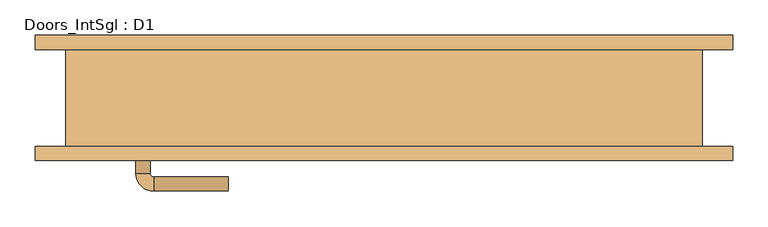
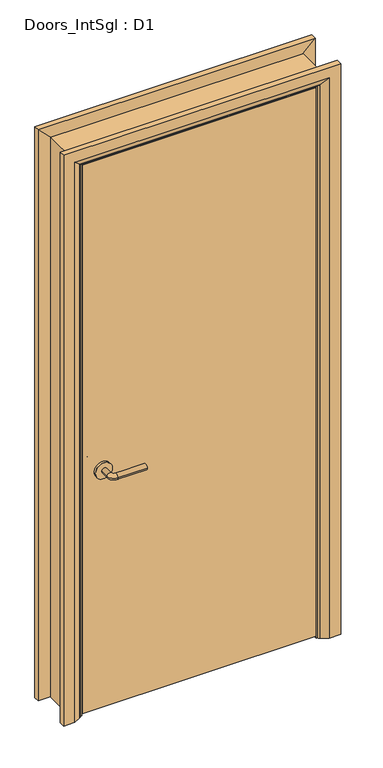
"""IFC4 building model written with IfcOpenShell, lengths in millimetres: door geometry, Doors_IntSgl : D1."""

from ifc_helpers import new_model, si_unit, point, frame, frame_2d, origin, place, context, project, spatial, polyline, circle_curve, ellipse_curve, trimmed, segment, composite_curve, outline, extrude, faceted_brep, source, transform, mapped, element, save
from ifc_brep_helpers import plane_surface, cylinder_surface, revolved_surface, advanced_brep


def doors_intsgl_d1_00c56c0f(model_context):
    return source(origin(), model_context, "Body", "SolidModel", [
        advanced_brep(
        [(-350.2, -22.58, 900.0), (-330.2, -22.58, 900.0), (-350.2, 7.42, 900.0), (-330.2, 7.42, 900.0), (-325.2, 12.42, 900.0), (-325.2, 32.42, 900.0), (-220.2, 32.42, 900.0), (-220.2, 12.42, 900.0)],
        [
            (0, 1, circle_curve(frame((-340.2, -22.58, 900.0), z_axis=(0.0, -1.0, 0.0), x_axis=(1.0, 0.0, 0.0)), 10.0)),
            (1, 0, circle_curve(frame((-340.2, -22.58, 900.0), z_axis=(0.0, -1.0, 0.0), x_axis=(1.0, 0.0, 0.0)), 10.0)),
            (0, 2),
            (2, 3, circle_curve(frame((-340.2, 7.42, 900.0), z_axis=(0.0, -1.0, 0.0), x_axis=(1.0, 0.0, 0.0)), 10.0)),
            (3, 1),
            (3, 2, circle_curve(frame((-340.2, 7.42, 900.0), z_axis=(0.0, -1.0, 0.0), x_axis=(1.0, 0.0, 0.0)), 10.0)),
            (4, 3, circle_curve(frame((-325.2, 7.42, 900.0), z_axis=(0.0, 0.0, 1.0), x_axis=(-1.0, 0.0, 0.0)), 5.0)),
            (2, 5, circle_curve(frame((-325.2, 7.42, 900.0), z_axis=(0.0, 0.0, -1.0), x_axis=(-1.0, 0.0, 0.0)), 25.0)),
            (5, 4, circle_curve(frame((-325.2, 22.42, 900.0), z_axis=(-1.0, 0.0, 0.0), x_axis=(0.0, -1.0, 0.0)), 10.0)),
            (4, 5, circle_curve(frame((-325.2, 22.42, 900.0), z_axis=(-1.0, 0.0, 0.0), x_axis=(0.0, -1.0, 0.0)), 10.0)),
            (6, 7, circle_curve(frame((-220.2, 22.42, 900.0), z_axis=(1.0, 0.0, 0.0), x_axis=(0.0, -1.0, 0.0)), 10.0)),
            (7, 6, circle_curve(frame((-220.2, 22.42, 900.0), z_axis=(1.0, 0.0, 0.0), x_axis=(0.0, -1.0, 0.0)), 10.0)),
            (5, 6),
            (7, 4),
        ],
        [
            plane_surface(frame((-340.2, -22.58, 900.0), z_axis=(0.0, -1.0, 0.0), x_axis=(0.0, 0.0, 1.0))),
            cylinder_surface(frame((-340.2, -22.58, 900.0), z_axis=(0.0, -1.0, 0.0), x_axis=(1.0, 0.0, 0.0)), 10.0),
            revolved_surface(trimmed(ellipse_curve(frame((-340.2, 7.42, 900.0), z_axis=(0.0, -1.0, 0.0), x_axis=(1.0, 0.0, 0.0)), 10.0, 10.0), [point((-350.2, 7.42, 900.0))], [point((-330.2, 7.42, 900.0))], True, "CARTESIAN"), (-325.2, 7.42, 900.0), (0.0, 0.0, -1.0)),
            revolved_surface(trimmed(ellipse_curve(frame((-340.2, 7.42, 900.0), z_axis=(0.0, -1.0, 0.0), x_axis=(1.0, 0.0, 0.0)), 10.0, 10.0), [point((-330.2, 7.42, 900.0))], [point((-350.2, 7.42, 900.0))], True, "CARTESIAN"), (-325.2, 7.42, 900.0), (0.0, 0.0, -1.0)),
            plane_surface(frame((-220.2, 22.42, 900.0), z_axis=(1.0, 0.0, 0.0), x_axis=(0.0, 0.0, 1.0))),
            cylinder_surface(frame((-325.2, 22.42, 900.0), z_axis=(-1.0, 0.0, 0.0), x_axis=(0.0, -1.0, 0.0)), 10.0),
        ],
        [
            (0, [[1, 2]]),
            (1, [[-1, 3, 4, 5]]),
            (1, [[-2, -5, 6, -3]]),
            (2, [[7, -4, 8, 9]]),
            (3, [[-8, -6, -7, 10]]),
            (4, [[11, 12]]),
            (5, [[-9, 13, -12, 14]]),
            (5, [[-10, -14, -11, -13]]),
        ],
    ),
        extrude(outline(composite_curve([segment(trimmed(circle_curve(frame_2d((900.0, -342.7)), 30.0), [point((900.0, -372.7))], [point((900.0, -312.7))], False, "CARTESIAN"), True, "CONTINUOUS"), segment(trimmed(circle_curve(frame_2d((900.0, -342.7)), 30.0), [point((900.0, -312.7))], [point((900.0, -372.7))], False, "CARTESIAN"), True, "CONTINUOUS")], self_intersect=False)), frame((0.0, -30.58, 0.0), z_axis=(0.0, 1.0, 0.0), x_axis=(0.0, 0.0, 1.0)), (0.0, 0.0, 1.0), 8.0),
        advanced_brep(
        [(-350.2, -76.58, 900.0), (-330.2, -76.58, 900.0), (-330.2, -106.58, 900.0), (-350.2, -106.58, 900.0), (-325.2, -111.58, 900.0), (-325.2, -131.58, 900.0), (-220.2, -131.58, 900.0), (-220.2, -111.58, 900.0)],
        [
            (0, 1, circle_curve(frame((-340.2, -76.58, 900.0), z_axis=(0.0, 1.0, 0.0), x_axis=(1.0, 0.0, 0.0)), 10.0)),
            (1, 0, circle_curve(frame((-340.2, -76.58, 900.0), z_axis=(0.0, 1.0, 0.0), x_axis=(1.0, 0.0, 0.0)), 10.0)),
            (1, 2),
            (2, 3, circle_curve(frame((-340.2, -106.58, 900.0), z_axis=(0.0, 1.0, 0.0), x_axis=(1.0, 0.0, 0.0)), 10.0)),
            (3, 0),
            (3, 2, circle_curve(frame((-340.2, -106.58, 900.0), z_axis=(0.0, 1.0, 0.0), x_axis=(1.0, 0.0, 0.0)), 10.0)),
            (4, 5, circle_curve(frame((-325.2, -121.58, 900.0), z_axis=(-1.0, 0.0, 0.0), x_axis=(0.0, 1.0, 0.0)), 10.0)),
            (5, 3, circle_curve(frame((-325.2, -106.58, 900.0), z_axis=(0.0, 0.0, -1.0), x_axis=(-1.0, 0.0, 0.0)), 25.0)),
            (2, 4, circle_curve(frame((-325.2, -106.58, 900.0), z_axis=(0.0, 0.0, 1.0), x_axis=(-1.0, 0.0, 0.0)), 5.0)),
            (5, 4, circle_curve(frame((-325.2, -121.58, 900.0), z_axis=(-1.0, 0.0, 0.0), x_axis=(0.0, 1.0, 0.0)), 10.0)),
            (6, 7, circle_curve(frame((-220.2, -121.58, 900.0), z_axis=(1.0, 0.0, 0.0), x_axis=(0.0, 1.0, 0.0)), 10.0)),
            (7, 6, circle_curve(frame((-220.2, -121.58, 900.0), z_axis=(1.0, 0.0, 0.0), x_axis=(0.0, 1.0, 0.0)), 10.0)),
            (4, 7),
            (6, 5),
        ],
        [
            plane_surface(frame((-340.2, -76.58, 900.0), z_axis=(0.0, 1.0, 0.0), x_axis=(0.0, 0.0, 1.0))),
            cylinder_surface(frame((-340.2, -76.58, 900.0), z_axis=(0.0, 1.0, 0.0), x_axis=(1.0, 0.0, 0.0)), 10.0),
            revolved_surface(trimmed(ellipse_curve(frame((-340.2, -106.58, 900.0), z_axis=(0.0, -1.0, 0.0), x_axis=(1.0, 0.0, 0.0)), 10.0, 10.0), [point((-350.2, -106.58, 900.0))], [point((-330.2, -106.58, 900.0))], True, "CARTESIAN"), (-325.2, -106.58, 900.0), (0.0, 0.0, -1.0)),
            revolved_surface(trimmed(ellipse_curve(frame((-340.2, -106.58, 900.0), z_axis=(0.0, -1.0, 0.0), x_axis=(1.0, 0.0, 0.0)), 10.0, 10.0), [point((-330.2, -106.58, 900.0))], [point((-350.2, -106.58, 900.0))], True, "CARTESIAN"), (-325.2, -106.58, 900.0), (0.0, 0.0, -1.0)),
            plane_surface(frame((-220.2, -121.58, 900.0), z_axis=(1.0, 0.0, 0.0), x_axis=(0.0, 0.0, 1.0))),
            cylinder_surface(frame((-325.2, -121.58, 900.0), z_axis=(-1.0, 0.0, 0.0), x_axis=(0.0, 1.0, 0.0)), 10.0),
        ],
        [
            (0, [[1, 2]]),
            (1, [[3, 4, 5, -2]]),
            (1, [[-5, 6, -3, -1]]),
            (2, [[7, 8, -4, 9]]),
            (3, [[10, -9, -6, -8]]),
            (4, [[11, 12]]),
            (5, [[13, -11, 14, -7]]),
            (5, [[-14, -12, -13, -10]]),
        ],
    ),
        extrude(outline(composite_curve([segment(trimmed(circle_curve(frame_2d((900.0, -342.7)), 30.0), [point((900.0, -372.7))], [point((900.0, -312.7))], False, "CARTESIAN"), True, "CONTINUOUS"), segment(trimmed(circle_curve(frame_2d((900.0, -342.7)), 30.0), [point((900.0, -312.7))], [point((900.0, -372.7))], False, "CARTESIAN"), True, "CONTINUOUS")], self_intersect=False)), frame((0.0, -76.58, 0.0), z_axis=(0.0, 1.0, 0.0), x_axis=(0.0, 0.0, 1.0)), (0.0, 0.0, 1.0), 8.0),
        extrude(outline(polyline([(415.2, -30.58), (415.2, -68.58), (-415.2, -68.58), (-415.2, -30.58), (415.2, -30.58)])), frame((0.0, 0.0, 8.0), z_axis=(0.0, 0.0, 1.0), x_axis=(1.0, 0.0, 0.0)), (0.0, 0.0, 1.0), 2060.0),
        advanced_brep(
        [(492.2, -88.58, 0.0), (452.2, -88.58, 0.0), (426.2, -74.58, 0.0), (422.2, -68.58, 0.0), (492.2, -68.58, 0.0), (492.2, -68.58, 2145.0), (492.2, -88.58, 2145.0), (422.2, -68.58, 2075.0), (-422.2, -68.58, 2075.0), (-422.2, -68.58, 0.0), (-492.2, -68.58, 0.0), (-492.2, -68.58, 2145.0), (426.2, -74.58, 2079.0), (452.2, -88.58, 2105.0), (-492.2, -88.58, 2145.0), (-492.2, -88.58, 0.0), (-452.2, -88.58, 0.0), (-452.2, -88.58, 2105.0), (-426.2, -74.58, 0.0), (-426.2, -74.58, 2079.0)],
        [
            (0, 1),
            (1, 2),
            (2, 3, circle_curve(frame((430.2, -67.58, 0.0), z_axis=(0.0, 0.0, -1.0), x_axis=(1.0, 0.0, 0.0)), 8.0622577)),
            (3, 4),
            (4, 0),
            (4, 5),
            (5, 6),
            (6, 0),
            (3, 7),
            (7, 8),
            (8, 9),
            (9, 10),
            (10, 11),
            (11, 5),
            (2, 12),
            (12, 7, ellipse_curve(frame((430.2, -67.58, 2083.0), z_axis=(0.7071067811865475, 0.0, -0.7071067811865475), x_axis=(-0.7071067811865474, 0.0, -0.7071067811865476)), 11.4017543, 8.0622577)),
            (1, 13),
            (13, 12),
            (6, 14),
            (14, 15),
            (15, 16),
            (16, 17),
            (17, 13),
            (10, 15),
            (14, 11),
            (9, 18, circle_curve(frame((-430.2, -67.58, 0.0), z_axis=(0.0, 0.0, -1.0), x_axis=(-1.0, 0.0, 0.0)), 8.0622577)),
            (18, 16),
            (19, 18),
            (8, 19, ellipse_curve(frame((-430.2, -67.58, 2083.0), z_axis=(-0.7071067811865475, 0.0, -0.7071067811865475), x_axis=(-0.7071067811865474, 0.0, 0.7071067811865476)), 11.4017543, 8.0622577)),
            (19, 17),
            (12, 19),
        ],
        [
            plane_surface(frame((422.2, -68.58, 0.0), z_axis=(0.0, 0.0, -1.0), x_axis=(0.0, 1.0, 0.0))),
            plane_surface(frame((492.2, -88.58, 0.0), z_axis=(1.0, 0.0, 0.0), x_axis=(0.0, 0.0, 1.0))),
            plane_surface(frame((492.2, -68.58, 0.0), z_axis=(0.0, 1.0, 0.0), x_axis=(0.0, 0.0, 1.0))),
            cylinder_surface(frame((430.2, -67.58, 0.0), z_axis=(0.0, 0.0, -1.0), x_axis=(1.0, 0.0, 0.0)), 8.0622577),
            plane_surface(frame((426.2, -74.58, 0.0), z_axis=(-0.4740998230350126, -0.880471099922178, 0.0), x_axis=(0.0, 0.0, 1.0))),
            plane_surface(frame((452.2, -88.58, 0.0), z_axis=(0.0, -1.0, 0.0), x_axis=(0.0, 0.0, 1.0))),
            plane_surface(frame((-492.2, -88.58, 2145.0), z_axis=(-1.0, 0.0, 0.0), x_axis=(0.0, 0.0, -1.0))),
            plane_surface(frame((-422.2, -68.58, 0.0), z_axis=(0.0, 0.0, -1.0), x_axis=(0.0, 1.0, 0.0))),
            cylinder_surface(frame((-430.2, -67.58, 2075.0), z_axis=(0.0, 0.0, 1.0), x_axis=(-1.0, 0.0, 0.0)), 8.0622577),
            plane_surface(frame((-426.2, -74.58, 2079.0), z_axis=(0.47409982303501824, -0.8804710999221749, 0.0), x_axis=(0.0, 0.0, -1.0))),
            plane_surface(frame((492.2, -88.58, 2145.0), z_axis=(0.0, 0.0, 1.0), x_axis=(-1.0, 0.0, 0.0))),
            cylinder_surface(frame((422.2, -67.58, 2083.0), z_axis=(1.0, 0.0, 0.0), x_axis=(0.0, 0.0, 1.0)), 8.0622577),
            plane_surface(frame((426.2, -74.58, 2079.0), z_axis=(0.0, -0.8804710999221764, -0.4740998230350154), x_axis=(-1.0, 0.0, 0.0))),
        ],
        [
            (0, [[1, 2, 3, 4, 5]]),
            (1, [[6, 7, 8, -5]]),
            (2, [[9, 10, 11, 12, 13, 14, -6, -4]]),
            (3, [[15, 16, -9, -3]]),
            (4, [[17, 18, -15, -2]]),
            (5, [[-8, 19, 20, 21, 22, 23, -17, -1]]),
            (6, [[-13, 24, -20, 25]]),
            (7, [[-24, -12, 26, 27, -21]]),
            (8, [[28, -26, -11, 29]]),
            (9, [[-22, -27, -28, 30]]),
            (10, [[-14, -25, -19, -7]]),
            (11, [[31, -29, -10, -16]]),
            (12, [[-23, -30, -31, -18]]),
        ],
    ),
        extrude(outline(polyline([(0.0, -398.2), (2051.0, -398.2), (2051.0, 398.2), (0.0, 398.2), (0.0, 417.2), (2070.0, 417.2), (2070.0, -417.2), (0.0, -417.2), (0.0, -398.2)])), frame((0.0, -28.58, 0.0), z_axis=(0.0, 1.0, 0.0), x_axis=(0.0, 0.0, 1.0)), (0.0, 0.0, 1.0), 32.0),
        advanced_brep(
        [(-492.2, 88.58, 0.0), (-452.2, 88.58, 0.0), (-426.2, 74.58, 0.0), (-422.2, 68.58, 0.0), (-492.2, 68.58, 0.0), (-492.2, 68.58, 2145.0), (-492.2, 88.58, 2145.0), (-422.2, 68.58, 2075.0), (-426.2, 74.58, 2079.0), (-452.2, 88.58, 2105.0), (492.2, 88.58, 0.0), (492.2, 68.58, 0.0), (422.2, 68.58, 0.0), (426.2, 74.58, 0.0), (452.2, 88.58, 0.0), (492.2, 88.58, 2145.0), (452.2, 88.58, 2105.0), (426.2, 74.58, 2079.0), (422.2, 68.58, 2075.0), (492.2, 68.58, 2145.0)],
        [
            (0, 1),
            (1, 2),
            (2, 3, circle_curve(frame((-430.2, 67.58, 0.0), z_axis=(0.0, 0.0, -1.0), x_axis=(-1.0, 0.0, 0.0)), 8.0622577)),
            (3, 4),
            (4, 0),
            (4, 5),
            (5, 6),
            (6, 0),
            (3, 7),
            (7, 5),
            (2, 8),
            (8, 7, ellipse_curve(frame((-430.2, 67.58, 2083.0), z_axis=(-0.7071067811865475, 0.0, -0.7071067811865475), x_axis=(0.7071067811865474, 0.0, -0.7071067811865476)), 11.4017543, 8.0622577)),
            (1, 9),
            (9, 8),
            (6, 9),
            (10, 11),
            (11, 12),
            (12, 13, circle_curve(frame((430.2, 67.58, 0.0), z_axis=(0.0, 0.0, -1.0), x_axis=(1.0, 0.0, 0.0)), 8.0622577)),
            (13, 14),
            (14, 10),
            (15, 10),
            (14, 16),
            (16, 15),
            (13, 17),
            (17, 16),
            (12, 18),
            (18, 17, ellipse_curve(frame((430.2, 67.58, 2083.0), z_axis=(0.7071067811865475, 0.0, -0.7071067811865475), x_axis=(0.7071067811865474, 0.0, 0.7071067811865476)), 11.4017543, 8.0622577)),
            (11, 19),
            (19, 18),
            (15, 19),
            (5, 19),
            (15, 6),
            (7, 18),
            (8, 17),
            (9, 16),
        ],
        [
            plane_surface(frame((-422.2, 141.3810989, 0.0), z_axis=(0.0, 0.0, -1.0), x_axis=(1.0, 0.0, 0.0))),
            plane_surface(frame((-492.2, 88.58, 0.0), z_axis=(-1.0, 0.0, 0.0), x_axis=(0.0, 0.0, 1.0))),
            plane_surface(frame((-492.2, 68.58, 0.0), z_axis=(0.0, -1.0, 0.0), x_axis=(0.0, 0.0, 1.0))),
            cylinder_surface(frame((-430.2, 67.58, 0.0), z_axis=(0.0, 0.0, -1.0), x_axis=(-1.0, 0.0, 0.0)), 8.0622577),
            plane_surface(frame((-426.2, 74.58, 0.0), z_axis=(0.4740998230350183, 0.8804710999221749, 0.0), x_axis=(0.0, 0.0, 1.0))),
            plane_surface(frame((-452.2, 88.58, 0.0), z_axis=(0.0, 1.0, 0.0), x_axis=(0.0, 0.0, 1.0))),
            plane_surface(frame((422.2, 141.3810989, 0.0), z_axis=(0.0, 0.0, -1.0), x_axis=(-1.0, 0.0, 0.0))),
            plane_surface(frame((452.2, 88.58, 2105.0), z_axis=(0.0, 1.0, 0.0), x_axis=(0.0, 0.0, -1.0))),
            plane_surface(frame((426.2, 74.58, 2079.0), z_axis=(-0.4740998230350183, 0.8804710999221749, 0.0), x_axis=(0.0, 0.0, -1.0))),
            cylinder_surface(frame((430.2, 67.58, 2075.0), z_axis=(0.0, 0.0, 1.0), x_axis=(1.0, 0.0, 0.0)), 8.0622577),
            plane_surface(frame((492.2, 68.58, 2145.0), z_axis=(0.0, -1.0, 0.0), x_axis=(0.0, 0.0, -1.0))),
            plane_surface(frame((492.2, 88.58, 2145.0), z_axis=(1.0, 0.0, 0.0), x_axis=(0.0, 0.0, -1.0))),
            plane_surface(frame((-492.2, 88.58, 2145.0), z_axis=(0.0, 0.0, 1.0), x_axis=(1.0, 0.0, 0.0))),
            plane_surface(frame((-492.2, 68.58, 2145.0), z_axis=(0.0, -1.0, 0.0), x_axis=(1.0, 0.0, 0.0))),
            cylinder_surface(frame((-422.2, 67.58, 2083.0), z_axis=(-1.0, 0.0, 0.0), x_axis=(0.0, 0.0, 1.0)), 8.0622577),
            plane_surface(frame((-426.2, 74.58, 2079.0), z_axis=(0.0, 0.8804710999221749, -0.4740998230350183), x_axis=(1.0, 0.0, 0.0))),
            plane_surface(frame((-452.2, 88.58, 2105.0), z_axis=(0.0, 1.0, 0.0), x_axis=(1.0, 0.0, 0.0))),
        ],
        [
            (0, [[1, 2, 3, 4, 5]]),
            (1, [[6, 7, 8, -5]]),
            (2, [[9, 10, -6, -4]]),
            (3, [[11, 12, -9, -3]]),
            (4, [[13, 14, -11, -2]]),
            (5, [[-8, 15, -13, -1]]),
            (6, [[16, 17, 18, 19, 20]]),
            (7, [[21, -20, 22, 23]]),
            (8, [[-22, -19, 24, 25]]),
            (9, [[-24, -18, 26, 27]]),
            (10, [[-26, -17, 28, 29]]),
            (11, [[-28, -16, -21, 30]]),
            (12, [[31, -30, 32, -7]]),
            (13, [[33, -29, -31, -10]]),
            (14, [[34, -27, -33, -12]]),
            (15, [[35, -25, -34, -14]]),
            (16, [[-32, -23, -35, -15]]),
        ],
    ),
        faceted_brep([(-417.2, -68.58, 0.0), (-449.2, -68.58, 0.0), (-449.2, 68.58, 0.0), (-417.2, 68.58, 0.0), (-417.2, 68.58, 2070.0), (-417.2, -68.58, 2070.0), (-449.2, 68.58, 2102.0), (-449.2, -68.58, 2102.0), (417.2, -68.58, 0.0), (417.2, 68.58, 0.0), (449.2, 68.58, 0.0), (449.2, -68.58, 0.0), (417.2, -68.58, 2070.0), (449.2, -68.58, 2102.0), (449.2, 68.58, 2102.0), (417.2, 68.58, 2070.0)], [[[0, 1, 2, 3]], [[3, 4, 5, 0]], [[2, 6, 4, 3]], [[1, 7, 6, 2]], [[0, 5, 7, 1]], [[8, 9, 10, 11]], [[12, 8, 11, 13]], [[13, 11, 10, 14]], [[14, 10, 9, 15]], [[15, 9, 8, 12]], [[4, 15, 12, 5]], [[6, 14, 15, 4]], [[7, 13, 14, 6]], [[5, 12, 13, 7]]]),
    ])


if __name__ == "__main__":
    model = new_model("IFC4")
    model_context = context("Model", 3, world=origin())
    ifc_project = project(units=[si_unit("LENGTHUNIT", "METRE", prefix="MILLI")], contexts=[model_context])
    site = spatial("IfcSite", under=ifc_project)
    building = spatial("IfcBuilding", under=site)
    placement = place(None, origin())
    doors_intsgl_d1_shape = doors_intsgl_d1_00c56c0f(model_context)
    element("IfcDoor", 1, ObjectType="Doors_IntSgl : D1", at=placement, inside=building, context=model_context, shape_type="MappedRepresentation", body=[
        mapped(doors_intsgl_d1_shape, transform((0.0, 0.0, 0.0), x_axis=(1.0, 0.0, 0.0), y_axis=(0.0, 1.0, 0.0), z_axis=(0.0, 0.0, 1.0))),
    ])
    save(model, "model.ifc")

# Revit data of these elements
# Type "Doors_IntSgl : D1"
#   Type Mark = "46"
#   Type Comments = "Internal Single"
#   Operation = "SingleSwingRight"
#   Manufacturer = "Revit"
#   Keynote = "L20"
#   Description = "Internal Single Door"
#   Analytic Construction = "Metal"
#   UnderCut = 8 mm
#   Tolerance = 2 mm
#   Thickness = 38 mm
#   Thermal Resistance (R) = 0.270117 (m²·K)/W
#   Structural Tolerance = 8 mm
#   StopDepth = 32 mm
#   Stop Thickness = 19 mm
#   Rough Width = 914.4 mm
#   Rough Height = 2110 mm
#   Height to Top Lock Rail = 1000 mm
#   Heat Transfer Coefficient (U) = 3.7021 W/(m²·K)
#   Handle Z Distance = 900 mm
#   Handle X Distance = 75 mm
#   Frame Thickness = 32 mm
#   Door Panel Width = 830.4 mm
#   Door Panel Thickness = 38 mm
#   Door Panel Offset = 0 mm
#   Height = 2110 mm
#   Width = 914.4 mm
#   Door Panel Height = 2060 mm
#   Architrave Setback = 5 mm
#   Vis - Ironmongery = yes
#   Material Ironmongery = Door - Handle
#   Material Frame = Door - Frame/Mullion (1)
#   Material Door = Door - Panel
#   Material Architrave = Door - Architrave
#   Visual Light Transmittance = 0
#   Solar Heat Gain Coefficient = 0
#   Function = (empty or 0)
#   Wall Closure = (empty or 0)
# Element 1 (IfcDoor, "Doors_IntSgl : D1")
#   Materials on its faces: "Door - Architrave", "Door - Handle", "Door - Frame/Mullion (1)", "Door - Panel"
# Materials
#   "Door - Handle": colour RGB 0 0 0, transparency 0, Keynote = "P21", Cost = 0
#   "Door - Frame/Mullion (1)": class "Wood", colour RGB 212 179 113, transparency 0, Keynote = "L20", Cost = 0
#   "Door - Panel": class "Wood", colour RGB 210 159 95, transparency 0, Keynote = "L20", Cost = 0
#   "Door - Architrave": class "Wood", colour RGB 154 90 5, transparency 0, Keynote = "P20", Cost = 0
